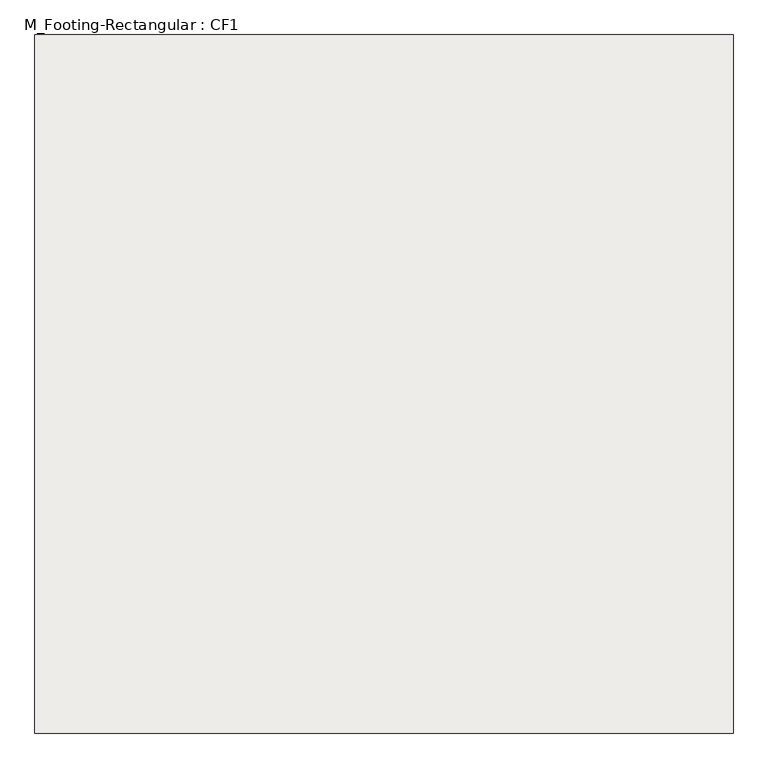
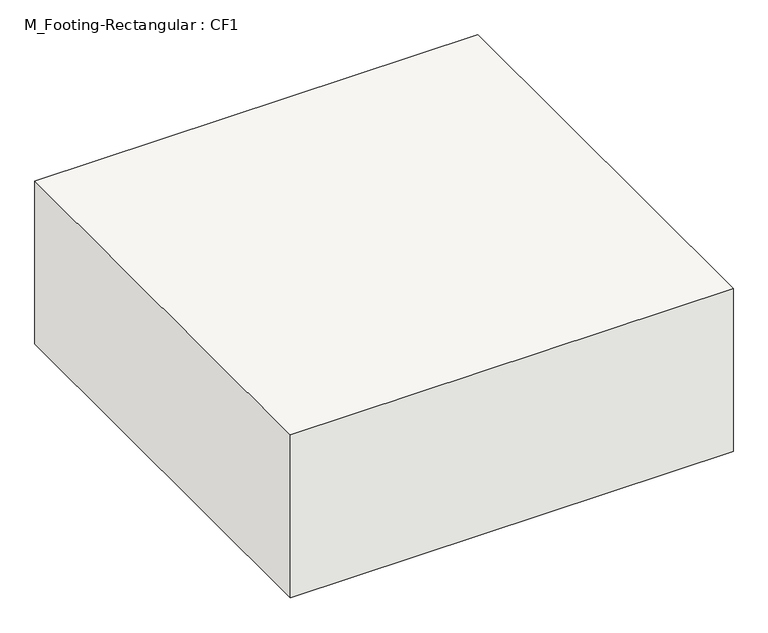
"""IFC4 building model written with IfcOpenShell, lengths in millimetres: slab geometry, M_Footing-Rectangular : CF1."""

from ifc_helpers import new_model, si_unit, frame, origin, place, context, project, spatial, polyline, outline, extrude, source, transform, mapped, element, save


def m_footing_rectangular_cf1_e8ad81a8(model_context):
    return source(origin(), model_context, "Body", "SweptSolid", [
        extrude(outline(polyline([(685.8, 685.8), (685.8, -685.8), (-685.8, -685.8), (-685.8, 685.8), (685.8, 685.8)])), frame((0.0, 0.0, -533.4), z_axis=(0.0, 0.0, 1.0), x_axis=(1.0, 0.0, 0.0)), (0.0, 0.0, 1.0), 533.4),
    ])


if __name__ == "__main__":
    model = new_model("IFC4")
    model_context = context("Model", 3, world=origin())
    ifc_project = project(units=[si_unit("LENGTHUNIT", "METRE", prefix="MILLI")], contexts=[model_context])
    site = spatial("IfcSite", under=ifc_project)
    building = spatial("IfcBuilding", under=site)
    placement = place(None, origin())
    m_footing_rectangular_cf1_shape = m_footing_rectangular_cf1_e8ad81a8(model_context)
    element("IfcSlab", 1, ObjectType="M_Footing-Rectangular : CF1", at=placement, inside=building, context=model_context, shape_type="MappedRepresentation", body=[
        mapped(m_footing_rectangular_cf1_shape, transform((0.0, 0.0, 0.0), x_axis=(1.0, 0.0, 0.0), y_axis=(0.0, 1.0, 0.0), z_axis=(0.0, 0.0, 1.0))),
    ])
    save(model, "model.ifc")

# Revit data of these elements
# Type "M_Footing-Rectangular : CF1"
#   Width = 1371.6 mm
#   Length = 1371.6 mm
#   Foundation Thickness = 533.4 mm
#   Structural Material [instance default] = Concrete, Cast-in-Place gray
#   Assembly Code = ""
# Element 1 (IfcSlab, "M_Footing-Rectangular : CF1")
#   Materials on its faces: "Concrete, Cast-in-Place gray"
# Materials
#   "Concrete, Cast-in-Place gray": class "Concrete", colour RGB 192 192 192, transparency 0, Description = "Cast-in-place concrete", Cost = 0
